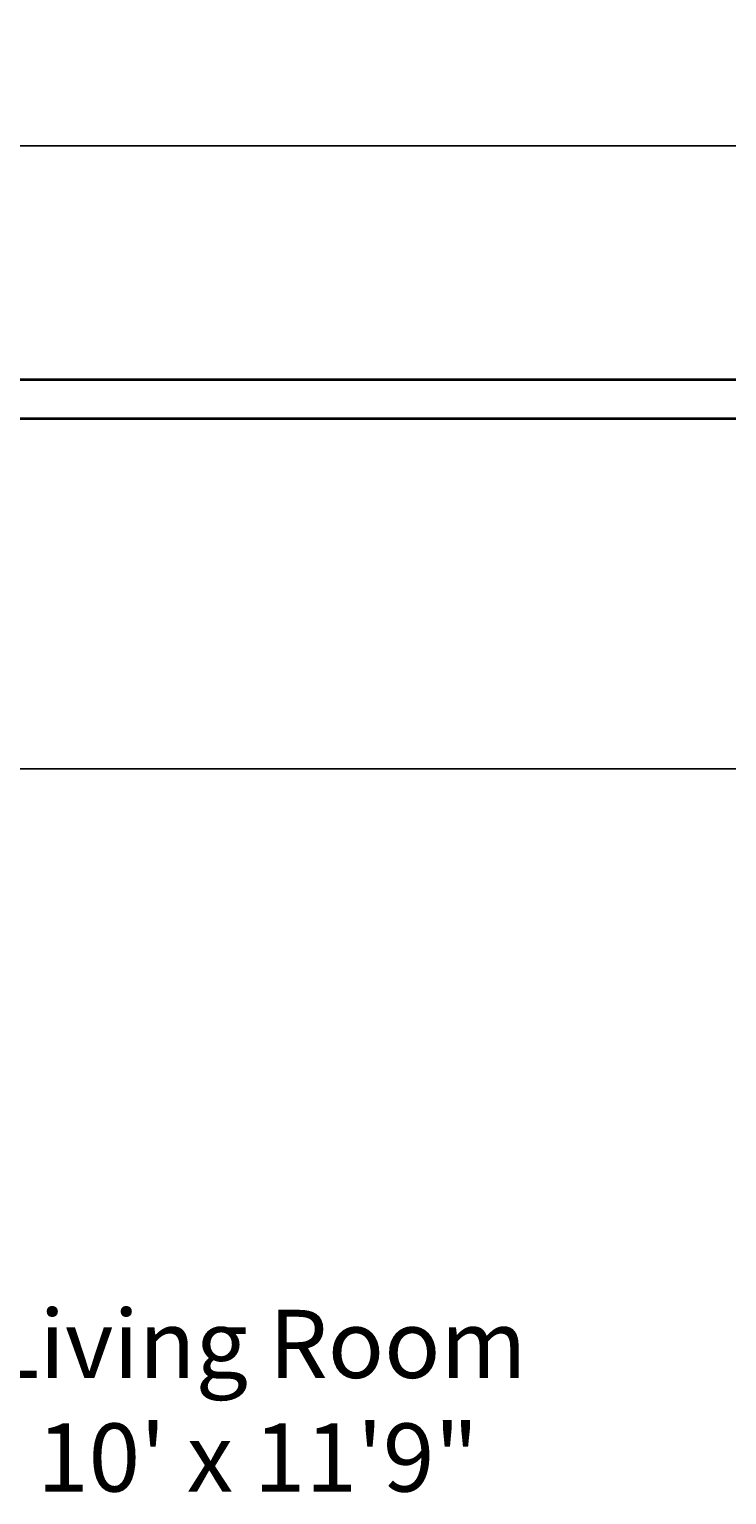
# Model space of a CAD drawing. Units: feet. Extents: x 105 to 1094, y -88 to 588.
# Tile 39 of 59: x 690 to 762, y 138 to 288. Entities that reach past the tile are written whole.
import ezdxf

# ---------------------------------------------------------------- set-up
doc = ezdxf.new("R2010")
doc.units = ezdxf.units.FT
doc.header["$MEASUREMENT"] = 0
for name, color, linetype, lineweight in [('A-ANNO-DIMS', 2, 'Continuous', 18), ('A-AREA-IDEN', 7, 'Continuous', 18), ('A-WALL', 7, 'Continuous', 35)]:
    doc.layers.add(name, color=color, linetype=linetype, lineweight=lineweight)
doc.styles.get("Standard").update_dxf_attribs({"font": 'arial.ttf'})
doc.dimstyles.get("Standard").update_dxf_attribs({"dimtxt": 0.18, "dimasz": 0.18, "dimexe": 0.18, "dimexo": 0.0625, "dimgap": 0.09, "dimtad": 0, "dimtih": 1, "dimtoh": 1, "dimdec": 4, "dimzin": 0, "dimdsep": 46, "dimtxsty": 'Standard', "dimcen": 0.09, "dimadec": 0, "dimazin": 0, "dimtfac": 1, "dimtdec": 4, "dimtofl": 0, "dimtmove": 0, "dimatfit": 3, "dimfxl": 1, "dimtolj": 1, "dimtzin": 0, "dimarcsym": 0})

# ---------------------------------------------------------------- blocks, each defined once
blk = doc.blocks.new('*D20')
at = {"layer": 'A-ANNO-DIMS', "color": 0, "lineweight": -2, "transparency": 16777216}
for p, q in [((150.69, 276.02), (150.69, -88.15)), ((1048.69, 276.02), (1048.69, -88.15)), ((150.87, -87.97), (599.4, -87.97)), ((1048.51, -87.97), (599.98, -87.97))]:
    blk.add_line(p, q, dxfattribs=at)
at = {"layer": 'A-ANNO-DIMS', "color": 0, "transparency": 16777216}
for points in [[(150.87, -87.94), (150.87, -88), (150.69, -87.97)], [(1048.51, -87.94), (1048.51, -88), (1048.69, -87.97)]]:
    blk.add_solid(points, dxfattribs=at)
at = {"layer": 'Defpoints', "color": 0, "transparency": 16777216}
for p in [(150.69, 276.08), (1048.69, 276.08), (1048.69, -87.97)]:
    blk.add_point(p, dxfattribs=at)
at = {"layer": 'A-ANNO-DIMS', "color": 0, "transparency": 16777216, "insert": (599.69, -87.97), "char_height": 0.18, "attachment_point": 5}
blk.add_mtext('\\A1;898', dxfattribs=at)
blk = doc.blocks.new('*D21')
at = {"layer": 'A-ANNO-DIMS', "color": 0, "lineweight": -2, "transparency": 16777216}
for p, q in [((849.63, 543.08), (105.46, 543.08)), ((105.64, 542.9), (105.64, 250.26)), ((105.64, -42.74), (105.64, 249.9)), ((849.63, -42.92), (105.46, -42.92))]:
    blk.add_line(p, q, dxfattribs=at)
at = {"layer": 'A-ANNO-DIMS', "color": 0, "transparency": 16777216}
for points in [[(105.61, 542.9), (105.67, 542.9), (105.64, 543.08)], [(105.61, -42.74), (105.67, -42.74), (105.64, -42.92)]]:
    blk.add_solid(points, dxfattribs=at)
at = {"layer": 'Defpoints', "color": 0, "transparency": 16777216}
for p in [(105.64, 543.08), (849.69, 543.08), (849.69, -42.92)]:
    blk.add_point(p, dxfattribs=at)
at = {"layer": 'A-ANNO-DIMS', "color": 0, "transparency": 16777216, "insert": (105.64, 250.08), "char_height": 0.18, "attachment_point": 5}
blk.add_mtext('\\A1;586', dxfattribs=at)
blk = doc.blocks.new('*D34')
at = {"layer": 'A-ANNO-DIMS', "color": 0, "lineweight": -2, "transparency": 16777216}
for p, q in [((552.75, 295.08), (1093.92, 295.08)), ((1093.74, 294.9), (1093.74, 253.76)), ((1093.74, 212.26), (1093.74, 253.4)), ((552.75, 212.08), (1093.92, 212.08))]:
    blk.add_line(p, q, dxfattribs=at)
at = {"layer": 'A-ANNO-DIMS', "color": 0, "transparency": 16777216}
for points in [[(1093.71, 294.9), (1093.77, 294.9), (1093.74, 295.08)], [(1093.71, 212.26), (1093.77, 212.26), (1093.74, 212.08)]]:
    blk.add_solid(points, dxfattribs=at)
at = {"layer": 'Defpoints', "color": 0, "transparency": 16777216}
for p in [(552.69, 295.08), (552.69, 212.08), (1093.74, 212.08)]:
    blk.add_point(p, dxfattribs=at)
at = {"layer": 'A-ANNO-DIMS', "color": 0, "transparency": 16777216, "insert": (1093.74, 253.58), "char_height": 0.18, "attachment_point": 5}
blk.add_mtext('\\A1;83', dxfattribs=at)
blk = doc.blocks.new('*D54')
at = {"layer": 'A-ANNO-DIMS', "color": 0, "lineweight": -2, "transparency": 16777216}
for p, q in [((294.75, 296.08), (1093.92, 296.08)), ((1093.74, 295.9), (1093.74, 286.26)), ((1093.74, 276.26), (1093.74, 285.9)), ((294.75, 276.08), (1093.92, 276.08))]:
    blk.add_line(p, q, dxfattribs=at)
at = {"layer": 'A-ANNO-DIMS', "color": 0, "transparency": 16777216}
for points in [[(1093.71, 295.9), (1093.77, 295.9), (1093.74, 296.08)], [(1093.71, 276.26), (1093.77, 276.26), (1093.74, 276.08)]]:
    blk.add_solid(points, dxfattribs=at)
at = {"layer": 'Defpoints', "color": 0, "transparency": 16777216}
for p in [(294.69, 296.08), (1093.74, 296.08), (294.69, 276.08)]:
    blk.add_point(p, dxfattribs=at)
at = {"layer": 'A-ANNO-DIMS', "color": 0, "transparency": 16777216, "insert": (1093.74, 286.08), "char_height": 0.18, "attachment_point": 5}
blk.add_mtext('\\A1;20', dxfattribs=at)

msp = doc.modelspace()

# ---------------------------------------------------------------- linework, layer by layer
at = {"layer": 'A-WALL'}
for p, q in [((646.6883, 252.0812), (772.6883, 252.0812)), ((646.6883, 252.0812), (828.6883, 252.0812)), ((646.6883, 248.0812), (828.6883, 248.0812)), ((646.6883, 248.0812), (772.6883, 248.0812))]:
    msp.add_line(p, q, dxfattribs=at)

# ---------------------------------------------------------------- texts
at = {"layer": 'A-AREA-IDEN', "insert": (664.3247, 137.8526), "char_height": 7, "attachment_point": 7}
msp.add_mtext_dynamic_manual_height_columns('\\pxqc;Living Room \\P10\' x 11\'9"', width=98.34246, gutter_width=1, heights=[0], dxfattribs=at)

# ---------------------------------------------------------------- dimensions: what is measured, and where the dimension line sits
at = {"layer": 'A-ANNO-DIMS'}
for base, p1, p2, picture, middle in [((105.6383, 543.0812), (849.6883, -42.9188), (849.6883, 543.0812), '*D21', (105.6383, 250.0812)), ((1093.7383, 296.0812), (294.6883, 276.0812), (294.6883, 296.0812), '*D54', (1093.7383, 286.0812)), ((1093.7383, 212.0812), (552.6883, 295.0812), (552.6883, 212.0812), '*D34', (1093.7383, 253.5812))]:
    dim = msp.add_linear_dim(base=base, p1=p1, p2=p2, angle=90, dimstyle='Standard', override={"dimdec": 0, "dimlfac": 1, "dimrnd": 0, "dimzin": 0, "dimdsep": 46, "dimlunit": 2}, dxfattribs=at)
    dim.commit()
    dim.dimension.update_dxf_attribs({"geometry": picture, "text_midpoint": middle})
dim = msp.add_linear_dim(base=(1048.6883, -87.9688), p1=(150.6883, 276.0812), p2=(1048.6883, 276.0812), dimstyle='Standard', override={"dimdec": 0, "dimlfac": 1, "dimrnd": 0, "dimzin": 0, "dimdsep": 46, "dimlunit": 2}, dxfattribs=at)
dim.commit()
dim.dimension.update_dxf_attribs({"geometry": '*D20', "text_midpoint": (599.6883, -87.9688)})

doc.saveas('drawing.dxf')
